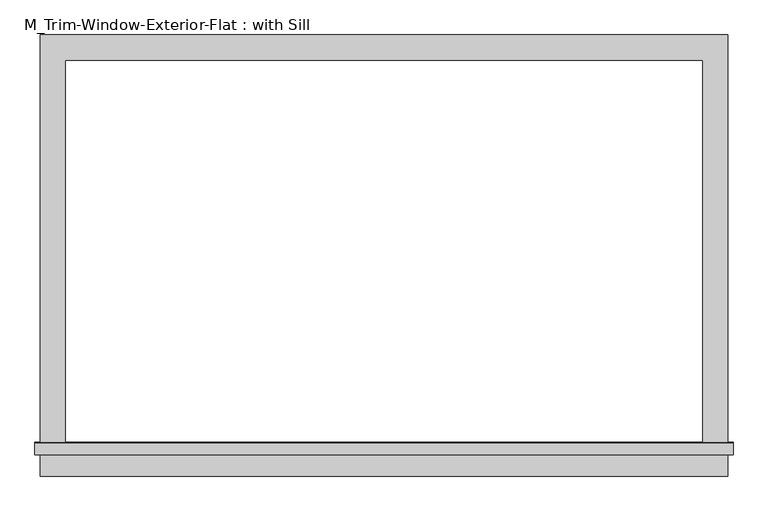
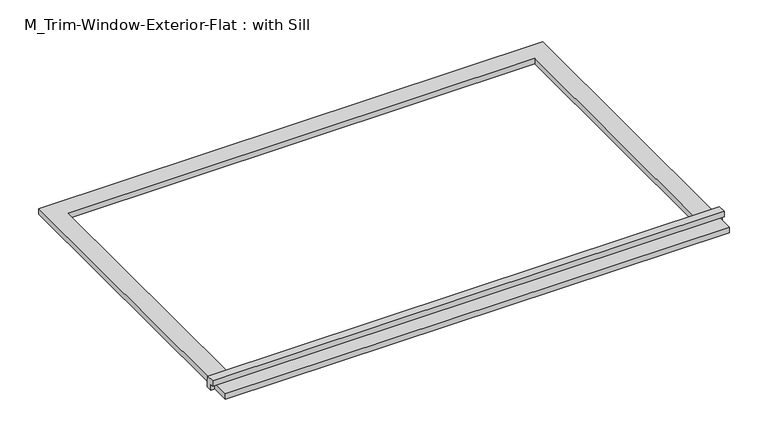
"""IFC4 building model written with IfcOpenShell, lengths in millimetres: proxy geometry, M_Trim-Window-Exterior-Flat : with Sill."""

from ifc_helpers import new_model, si_unit, frame, origin, origin_with_axes, place, context, project, spatial, polyline, outline, extrude, source, transform, mapped, element, save


def m_trim_window_exterior_flat_with_sill_e3533f3c(model_context):
    return source(origin(), model_context, "Body", "SweptSolid", [
        extrude(outline(polyline([(822.0, -934.8323709), (822.0, -994.8323709), (-822.0, -994.8323709), (-822.0, -934.8323709), (822.0, -934.8323709)])), origin_with_axes(), (0.0, 0.0, 1.0), 19.05),
        extrude(outline(polyline([(-944.4, 38.1), (-916.8580645, 38.1), (-914.4, 19.05), (-914.4, 0.0), (-934.8323709, 0.0), (-934.8323709, 19.05), (-944.4, 19.05), (-944.4, 38.1)])), frame((-834.7, 0.0, 0.0), z_axis=(1.0, 0.0, 0.0), x_axis=(0.0, 1.0, 0.0)), (0.0, 0.0, 1.0), 1669.4),
        extrude(outline(polyline([(-822.0, 60.0), (822.0, 60.0), (822.0, -914.4), (762.0, -914.4), (762.0, 0.0), (-762.0, 0.0), (-762.0, -914.4), (-822.0, -914.4), (-822.0, 60.0)])), origin_with_axes(), (0.0, 0.0, 1.0), 19.05),
    ])


if __name__ == "__main__":
    model = new_model("IFC4")
    model_context = context("Model", 3, world=origin())
    ifc_project = project(units=[si_unit("LENGTHUNIT", "METRE", prefix="MILLI")], contexts=[model_context])
    site = spatial("IfcSite", under=ifc_project)
    building = spatial("IfcBuilding", under=site)
    placement = place(None, origin())
    m_trim_window_exterior_flat_with_sill_shape = m_trim_window_exterior_flat_with_sill_e3533f3c(model_context)
    element("IfcBuildingElementProxy", 1, Name="M_Trim-Window-Exterior-Flat : with Sill", ObjectType="M_Trim-Window-Exterior-Flat : with Sill", at=placement, inside=building, context=model_context, shape_type="MappedRepresentation", body=[
        mapped(m_trim_window_exterior_flat_with_sill_shape, transform((0.0, 0.0, 0.0), x_axis=(1.0, 0.0, 0.0), y_axis=(0.0, 1.0, 0.0), z_axis=(0.0, 0.0, 1.0))),
    ])
    save(model, "model.ifc")

# Revit data of these elements
# Type "M_Trim-Window-Exterior-Flat : with Sill"
#   Trim Width = 0' - 2.3622"
#   Trim Thickness_Picture Frame = 0' - 1.1811"
#   Trim Thickness_with Sill = 0' - 0 3/4"
#   Sill Thickness = 0' - 1.1811"
#   Opening Width [instance default] = 1' - 11.62205"
#   Opening Height [instance default] = 2' - 11.43307"
#   Default Elevation = 3' - 11.24409"
#   Sill = yes
#   Picture Frame = no
#   Trim Material [instance default] = none
# Element 1 (IfcBuildingElementProxy, "M_Trim-Window-Exterior-Flat : with Sill")
#   Opening Width = 5' - 0"
#   Opening Height = 3' - 0"
#   Trim Material = Clad - White
#   Materials on its faces: "Clad - White"
# Materials
#   "Clad - White": class "Wood", colour RGB 242 242 238, transparency 0, Cost = 0
